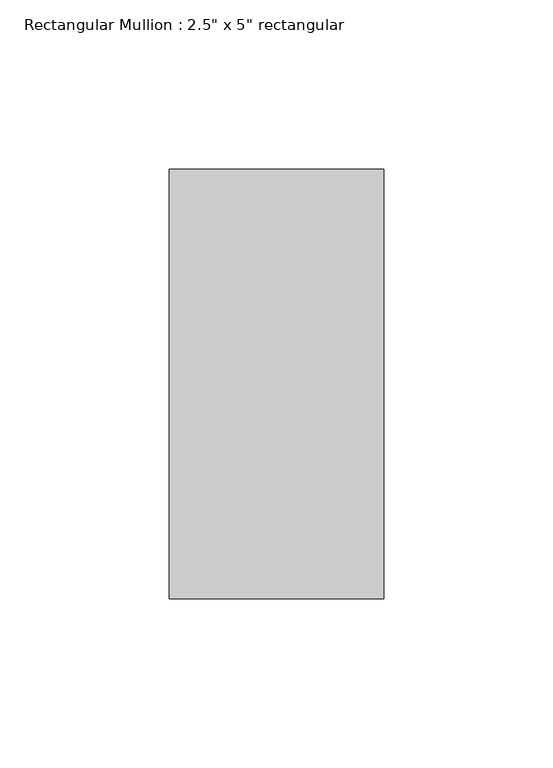
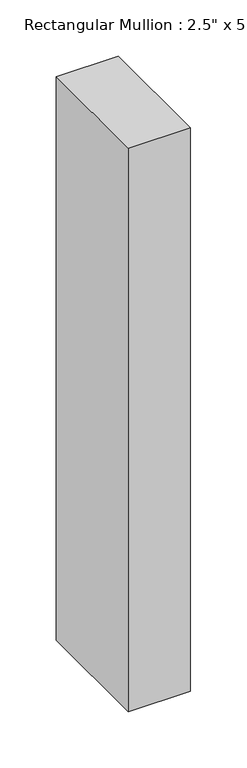
"""IFC4 building model written with IfcOpenShell, lengths in millimetres: member geometry."""

from ifc_helpers import new_model, si_unit, frame, origin, place, context, project, spatial, polyline, outline, extrude, source, transform, mapped, element, save


def member_47bfaf8a(model_context):
    return source(origin(), model_context, "Body", "SweptSolid", [
        extrude(outline(polyline([(0.0, 63.5), (0.0, -63.5), (-63.5, -63.5), (-63.5, 63.5), (0.0, 63.5)])), frame((0.0, 0.0, -609.6), z_axis=(0.0, 0.0, 1.0), x_axis=(1.0, 0.0, 0.0)), (0.0, 0.0, 1.0), 609.6),
    ])


if __name__ == "__main__":
    model = new_model("IFC4")
    model_context = context("Model", 3, world=origin())
    ifc_project = project(units=[si_unit("LENGTHUNIT", "METRE", prefix="MILLI")], contexts=[model_context])
    site = spatial("IfcSite", under=ifc_project)
    building = spatial("IfcBuilding", under=site)
    placement = place(None, origin())
    member_shape = member_47bfaf8a(model_context)
    element("IfcMember", 1, ObjectType="Rectangular Mullion : 2.5\" x 5\" rectangular", at=placement, inside=building, context=model_context, shape_type="MappedRepresentation", body=[
        mapped(member_shape, transform((0.0, 0.0, 0.0), x_axis=(1.0, 0.0, 0.0), y_axis=(0.0, 1.0, 0.0), z_axis=(0.0, 0.0, 1.0))),
    ])
    save(model, "model.ifc")

# Revit data of these elements
# Type "Rectangular Mullion : 2.5\" x 5\" rectangular"
#   built-in parameter 1007304 = 0.416667 (stored number, unit not read)
#   built-in parameter 1007301 = 0.104167 (stored number, unit not read)
#   built-in parameter 1007300 = 0.104167 (stored number, unit not read)
# Element 1 (IfcMember, "Rectangular Mullion : 2.5\" x 5\" rectangular")
#   Materials on its faces: "metal black"
# Materials
#   "metal black": class "Generic", colour RGB 120 120 120, transparency 0, Cost = 0
